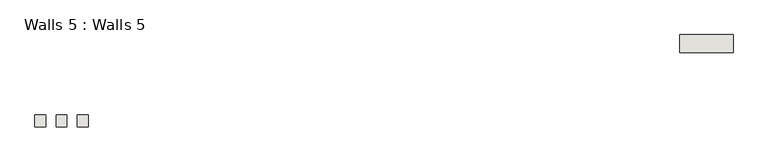
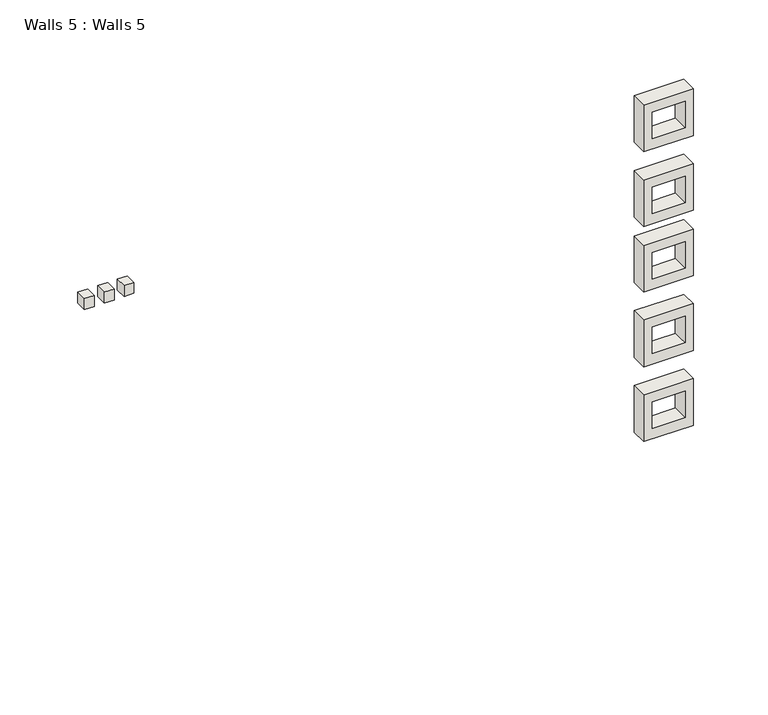
"""IFC4 building model written with IfcOpenShell, lengths in millimetres: wall geometry, Walls 5 : Walls 5."""

from ifc_helpers import new_model, si_unit, frame, origin, place, context, project, spatial, polyline, outline, extrude, source, transform, mapped, element, save


def walls_5_walls_5_6bae5a5a(model_context):
    return source(origin(), model_context, "Body", "SweptSolid", [
        extrude(outline(polyline([(-10660.5183714, -1444.1710271), (-10812.9183714, -1444.1710271), (-10812.9183714, -1269.1895946), (-10660.5183714, -1269.1895946), (-10660.5183714, -1444.1710271)])), frame((0.0, 0.0, 8165.6345389), z_axis=(0.0, 0.0, 1.0), x_axis=(1.0, 0.0, 0.0)), (0.0, 0.0, 1.0), 177.8),
        extrude(outline(polyline([(-10355.7183714, -1444.1710271), (-10508.1183714, -1444.1710271), (-10508.1183714, -1269.1895946), (-10355.7183714, -1269.1895946), (-10355.7183714, -1444.1710271)])), frame((0.0, 0.0, 8165.6345389), z_axis=(0.0, 0.0, 1.0), x_axis=(1.0, 0.0, 0.0)), (0.0, 0.0, 1.0), 177.8),
        extrude(outline(polyline([(-10050.9183714, -1444.1710271), (-10203.3183714, -1444.1710271), (-10203.3183714, -1269.1895946), (-10050.9183714, -1269.1895946), (-10050.9183714, -1444.1710271)])), frame((0.0, 0.0, 8165.6345389), z_axis=(0.0, 0.0, 1.0), x_axis=(1.0, 0.0, 0.0)), (0.0, 0.0, 1.0), 177.8),
        extrude(outline(polyline([(7620.0, -819.5999291), (7620.0, -1581.5999291), (6858.0, -1581.5999291), (6858.0, -819.5999291), (7620.0, -819.5999291)]), holes=[polyline([(7459.6528237, -943.4239156), (7027.8528237, -943.4239156), (7027.8528237, -1451.4239156), (7459.6528237, -1451.4239156), (7459.6528237, -943.4239156)])]), frame((0.0, -375.7099629, 0.0), z_axis=(0.0, 1.0, 0.0), x_axis=(0.0, 0.0, 1.0)), (0.0, 0.0, 1.0), 254.0),
        extrude(outline(polyline([(6400.8, -819.5999291), (6400.8, -1581.5999291), (5638.8, -1581.5999291), (5638.8, -819.5999291), (6400.8, -819.5999291)]), holes=[polyline([(6240.4528237, -943.4239156), (5808.6528237, -943.4239156), (5808.6528237, -1451.4239156), (6240.4528237, -1451.4239156), (6240.4528237, -943.4239156)])]), frame((0.0, -375.7099629, 0.0), z_axis=(0.0, 1.0, 0.0), x_axis=(0.0, 0.0, 1.0)), (0.0, 0.0, 1.0), 254.0),
        extrude(outline(polyline([(5334.0, -819.5999291), (5334.0, -1581.5999291), (4572.0, -1581.5999291), (4572.0, -819.5999291), (5334.0, -819.5999291)]), holes=[polyline([(5173.6528237, -943.4239156), (4741.8528237, -943.4239156), (4741.8528237, -1451.4239156), (5173.6528237, -1451.4239156), (5173.6528237, -943.4239156)])]), frame((0.0, -375.7099629, 0.0), z_axis=(0.0, 1.0, 0.0), x_axis=(0.0, 0.0, 1.0)), (0.0, 0.0, 1.0), 254.0),
        extrude(outline(polyline([(4114.8, -819.5999291), (4114.8, -1581.5999291), (3352.8, -1581.5999291), (3352.8, -819.5999291), (4114.8, -819.5999291)]), holes=[polyline([(3954.4528237, -943.4239156), (3522.6528237, -943.4239156), (3522.6528237, -1451.4239156), (3954.4528237, -1451.4239156), (3954.4528237, -943.4239156)])]), frame((0.0, -375.7099629, 0.0), z_axis=(0.0, 1.0, 0.0), x_axis=(0.0, 0.0, 1.0)), (0.0, 0.0, 1.0), 254.0),
        extrude(outline(polyline([(2895.6, -819.5999291), (2895.6, -1581.5999291), (2133.6, -1581.5999291), (2133.6, -819.5999291), (2895.6, -819.5999291)]), holes=[polyline([(2735.2528237, -943.4239156), (2303.4528237, -943.4239156), (2303.4528237, -1451.4239156), (2735.2528237, -1451.4239156), (2735.2528237, -943.4239156)])]), frame((0.0, -375.7099629, 0.0), z_axis=(0.0, 1.0, 0.0), x_axis=(0.0, 0.0, 1.0)), (0.0, 0.0, 1.0), 254.0),
    ])


if __name__ == "__main__":
    model = new_model("IFC4")
    model_context = context("Model", 3, world=origin())
    ifc_project = project(units=[si_unit("LENGTHUNIT", "METRE", prefix="MILLI")], contexts=[model_context])
    site = spatial("IfcSite", under=ifc_project)
    building = spatial("IfcBuilding", under=site)
    placement = place(None, origin())
    walls_5_walls_5_shape = walls_5_walls_5_6bae5a5a(model_context)
    element("IfcWall", 1, ObjectType="Walls 5 : Walls 5", at=placement, inside=building, context=model_context, shape_type="MappedRepresentation", body=[
        mapped(walls_5_walls_5_shape, transform((0.0, 0.0, 0.0), x_axis=(1.0, 0.0, 0.0), y_axis=(0.0, 1.0, 0.0), z_axis=(0.0, 0.0, 1.0))),
    ])
    save(model, "model.ifc")

# Revit data of these elements
# Element 1 (IfcWall, "Walls 5 : Walls 5")
#   Materials on its faces: "Default Wall"
# Materials
#   "Default Wall": colour RGB 128 128 128, transparency 0
